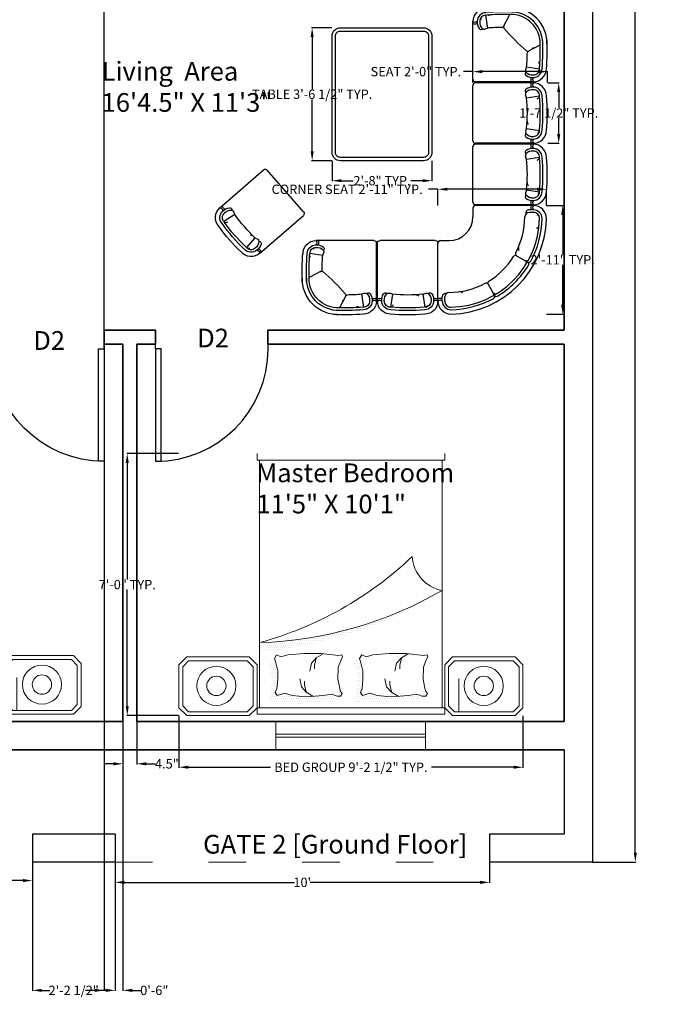
# Model space of a CAD drawing. Units: inches. Extents: x 593 to 1000, y 91 to 964.
# Tile 2 of 4: x 795 to 1000, y 91 to 406. Entities that reach past the tile are written whole.
import ezdxf

# ---------------------------------------------------------------- set-up
doc = ezdxf.new("R2010")
doc.units = ezdxf.units.IN
doc.header["$MEASUREMENT"] = 0
doc.linetypes.add('ACAD_ISO03W100', pattern=[30, 12, -18])
for name, color, linetype, lineweight in [('A-ANNO-DIMS', 2, 'Continuous', 13), ('A-ANNO-TEXT', 7, 'Continuous', 18), ('A-AREA-IDEN', 7, 'Continuous', 18), ('A-DOOR', 4, 'Continuous', 25), ('A-GLAZ', 4, 'Continuous', 18), ('A-WALL', 7, 'Continuous', 35), ('C-PROP', 7, 'Continuous', 30), ('C-SITE-GATE', 7, 'ACAD_ISO03W100', 18), ('FUR', 8, 'Continuous', 18)]:
    doc.layers.add(name, color=color, linetype=linetype, lineweight=lineweight)
doc.layers.add('ID-LOOSE', color=31, linetype='Continuous')
doc.layers.add('ID-LOOSE2', color=8, linetype='Continuous')
doc.styles.get("Standard").update_dxf_attribs({"font": 'arial.ttf'})
doc.dimstyles.get("Standard").update_dxf_attribs({"dimtxt": 3, "dimasz": 3, "dimexe": 0.18, "dimexo": 0.0625, "dimgap": 0.09, "dimtad": 0, "dimtih": 1, "dimtoh": 1, "dimdec": 1, "dimzin": 0, "dimdsep": 46, "dimlunit": 3, "dimtxsty": 'Standard', "dimcen": 0.09, "dimadec": 0, "dimazin": 0, "dimtfac": 1, "dimtdec": 1, "dimtofl": 0, "dimtmove": 0, "dimatfit": 3, "dimfxl": 1, "dimtolj": 1, "dimtzin": 0, "dimarcsym": 0})
pattern_1 = [(360, (-204.55691, -125.780183), (0.0079375, 0.015875), [0, -0.015875])]

# ---------------------------------------------------------------- blocks, each defined once
blk = doc.blocks.new('*U5')
for p, q in [((0, 0), (0, 6)), ((36, 0), (36, 6))]:
    blk.add_line(p, q)
blk.add_lwpolyline([(0, 0), (0, -36), (1.75, -36), (1.75, 0)], close=True)
blk.add_arc((0, 0), 36, 270, 0)
blk = doc.blocks.new('A$C9d18b682')
h = blk.add_hatch()
h.set_pattern_fill('DOTS', color=256, scale=0.01, style=0)
h.set_pattern_definition(pattern_1)
h.paths.add_polyline_path([(1.2038, 1.8915), (1.1915, 1.9099), (1.1638, 1.9099), (1.1238, 1.8945), (1.0562, 1.9068), (0.927, 1.916), (0.8193, 1.9068), (0.7639, 1.8884), (0.7055, 1.9068), (0.6901, 1.8822), (0.7024, 1.8546), (0.7086, 1.7839), (0.7086, 1.7163), (0.6932, 1.6548), (0.6839, 1.621), (0.6993, 1.5933), (0.7332, 1.6087), (0.7433, 1.6057), (0.7585, 1.6664), (0.7585, 1.734), (0.7523, 1.8047), (0.74, 1.8324), (0.7554, 1.857), (0.8139, 1.8385), (0.8692, 1.857), (0.9769, 1.8662), (1.1061, 1.857), (1.1738, 1.8447), (1.1846, 1.8488), (1.1884, 1.8699)])
h.paths.add_polyline_path([(1.8571, 1.8915), (1.8448, 1.9099), (1.8171, 1.9099), (1.7771, 1.8945), (1.7095, 1.9068), (1.5803, 1.916), (1.4726, 1.9068), (1.4172, 1.8884), (1.3588, 1.9068), (1.3434, 1.8822), (1.3557, 1.8546), (1.3618, 1.7839), (1.3618, 1.7163), (1.3465, 1.6548), (1.3372, 1.621), (1.3526, 1.5933), (1.3865, 1.6087), (1.3966, 1.6057), (1.4118, 1.6664), (1.4118, 1.734), (1.4056, 1.8047), (1.3933, 1.8324), (1.4087, 1.857), (1.4672, 1.8385), (1.5225, 1.857), (1.6302, 1.8662), (1.7594, 1.857), (1.8271, 1.8447), (1.8379, 1.8488), (1.8417, 1.8699)])
h = blk.add_hatch()
h.set_pattern_fill('DOTS', color=256, scale=0.01, style=0)
h.set_pattern_definition(pattern_1)
h.paths.add_polyline_path([(0.62, 1.5186), (0.62, 1.45, -0.124273), (2.02, 1.05, 0.122563)])
for p, q in [((2.04, 2), (0.6, 2)), ((0.6, 1.95), (0.6, 2)), ((2.04, 2), (2.04, 1.95)), ((2.1476, 1.9789), (2.1476, 1.7289)), ((2.04, 1.95), (0.6, 1.95)), ((0.62, 0.05), (0.62, 1.95)), ((2.02, 1.95), (2.02, 0.05)), ((2.04, 0.05), (0.6, 0.05)), ((0.6, 0), (0.6, 0.05)), ((2.04, 0.05), (2.04, 0))]:
    blk.add_line(p, q)
for points in [[(0.06, 1.56), (0.54, 1.56), (0.6, 1.62), (0.6, 1.95), (0.54, 2.01), (0.06, 2.01), (0, 1.95), (0, 1.62)], [(0.075, 1.59), (0.525, 1.59), (0.57, 1.635), (0.57, 1.935), (0.525, 1.98), (0.075, 1.98), (0.03, 1.935), (0.03, 1.635)], [(2.1, 1.56), (2.58, 1.56), (2.64, 1.62), (2.64, 1.95), (2.58, 2.01), (2.1, 2.01), (2.04, 1.95), (2.04, 1.62)], [(2.115, 1.59), (2.565, 1.59), (2.61, 1.635), (2.61, 1.935), (2.565, 1.98), (2.115, 1.98), (2.07, 1.935), (2.07, 1.635)]]:
    blk.add_lwpolyline(points, close=True)
for points in [[(0.8139, 1.8385), (0.7554, 1.857), (0.74, 1.8324), (0.7523, 1.8047), (0.7585, 1.734), (0.7585, 1.6664), (0.7431, 1.6049), (0.7339, 1.5711), (0.7493, 1.5434), (0.7831, 1.5588), (0.8354, 1.5434), (0.9615, 1.5342), (1.0907, 1.5342), (1.2261, 1.5496), (1.2507, 1.5434), (1.2568, 1.5588), (1.2445, 1.5834), (1.223, 1.6387), (1.2199, 1.7309), (1.2322, 1.7863), (1.2384, 1.8201), (1.2538, 1.8416), (1.2414, 1.86), (1.2138, 1.86), (1.1738, 1.8447), (1.1061, 1.857), (0.9769, 1.8662), (0.8692, 1.857), (0.8139, 1.8385)], [(1.0292, 1.86), (0.9769, 1.8293), (0.94, 1.7893), (0.9277, 1.7279)], [(0.9769, 1.8262), (0.9646, 1.777), (0.9646, 1.7463)], [(1.4672, 1.8385), (1.4087, 1.857), (1.3933, 1.8324), (1.4056, 1.8047), (1.4118, 1.734), (1.4118, 1.6664), (1.3964, 1.6049), (1.3872, 1.5711), (1.4026, 1.5434), (1.4364, 1.5588), (1.4887, 1.5434), (1.6148, 1.5342), (1.744, 1.5342), (1.8794, 1.5496), (1.904, 1.5434), (1.9101, 1.5588), (1.8978, 1.5834), (1.8763, 1.6387), (1.8732, 1.7309), (1.8855, 1.7863), (1.8917, 1.8201), (1.907, 1.8416), (1.8947, 1.86), (1.8671, 1.86), (1.8271, 1.8447), (1.7594, 1.857), (1.6302, 1.8662), (1.5225, 1.857), (1.4672, 1.8385)], [(1.6825, 1.86), (1.6302, 1.8293), (1.5933, 1.7893), (1.581, 1.7279)], [(1.6302, 1.8262), (1.6179, 1.777), (1.6179, 1.7463)], [(1.1061, 1.5373), (1.0538, 1.568), (1.0169, 1.608), (1.0046, 1.6695)], [(1.7594, 1.5373), (1.7071, 1.568), (1.6702, 1.608), (1.6579, 1.6695)], [(1.0538, 1.5711), (1.0415, 1.6203), (1.0415, 1.651)], [(1.7071, 1.5711), (1.6948, 1.6203), (1.6948, 1.651)]]:
    blk.add_lwpolyline(points)
for centre, radius in [((0.288, 1.782), 0.15), ((2.3392, 1.782), 0.15), ((0.288, 1.782), 0.0743), ((2.3392, 1.782), 0.0743)]:
    blk.add_circle(centre, radius)
for centre, radius, start, end in [((0.5277, -1.5229), 2.9743, 59.8866, 88.22261), ((-0.1045, -1.2025), 2.7497, 46.43667, 74.72336), ((2.0704, 0.7742), 0.2804, 100.35432, 176.78617)]:
    blk.add_arc(centre, radius, start, end)
blk = doc.blocks.new('A$C68294616')
at = {"layer": 'ID-LOOSE'}
for p, q in [((0.372, -0.31), (0.372, 0.36)), ((0.402, 0.39), (1.042, 0.39)), ((1.072, -0.31), (1.072, 0.36)), ((0.545, -0.231), (0.511, -0.219)), ((0.899, -0.231), (0.933, -0.219))]:
    blk.add_line(p, q, dxfattribs=at)
for centre, radius, start, end in [((0.402, 0.36), 0.03, 90, 180), ((1.042, 0.36), 0.03, 360, 90), ((0.554, -0.3), 0.133, 146.0897, 185.6132), ((0.465, -0.24), 0.025, 62.9608, 146.0897), ((0.452, -0.265), 0.0532, 51.0017, 62.9608), ((0.502, -0.242), 0.025, 70, 132.0066), ((0.942, -0.242), 0.025, 47.9934, 110), ((0.992, -0.265), 0.0532, 117.0392, 128.9983), ((0.979, -0.24), 0.025, 33.9103, 117.0392), ((0.89, -0.3), 0.133, 354.3868, 33.9103), ((0.397, -0.346), 0.0662, 67.8298, 112.1702), ((0.522, -0.31), 0.15, 180, 271.1754), ((0.522, -0.31), 0.1, 180, 271.1754), ((0.722, 1.538), 1.778, 264.2835, 275.7165), ((0.628, -0.286), 0.0481, 90.6237, 136.1803), ((0.922, -0.31), 0.15, 268.8246, 360), ((0.922, -0.31), 0.1, 268.8246, 360), ((1.047, -0.346), 0.0662, 67.8298, 112.1702), ((0.529, -0.332), 0.0481, 216.0775, 261.6341), ((0.722, 1.538), 1.958, 264.2835, 275.7165), ((0.933, -0.336), 0.0481, 201.2156, 246.7721), ((0.722, 1.538), 2.008, 264.2835, 275.7165)]:
    blk.add_arc(centre, radius, start, end, dxfattribs=at)
at = {"layer": 'ID-LOOSE2'}
for p, q in [((0.545, -0.231), (0.522, -0.38)), ((0.899, -0.231), (0.922, -0.38))]:
    blk.add_line(p, q, dxfattribs=at)
for centre, radius, start, end in [((0.554, -0.3), 0.103, 132.0066, 185.6132), ((0.89, -0.3), 0.103, 354.3868, 47.9934), ((0.397, -0.336), 0.0362, 46.3972, 133.6028), ((0.522, -0.31), 0.07, 180, 271.1754), ((0.922, -0.31), 0.07, 268.8246, 360), ((1.047, -0.336), 0.0362, 46.3972, 133.6028), ((0.722, 1.538), 1.928, 264.2835, 275.7165)]:
    blk.add_arc(centre, radius, start, end, dxfattribs=at)
blk = doc.blocks.new('A$C68FE3AF0')
at = {"layer": 'ID-LOOSE'}
for p, q in [((0.372, -0.31), (0.372, 0.36)), ((0.402, 0.39), (1.072, 0.39)), ((0.993, 0.217), (0.981, 0.251)), ((0.545, -0.231), (0.511, -0.219))]:
    blk.add_line(p, q, dxfattribs=at)
for centre, radius, start, end in [((0.402, 0.36), 0.03, 90, 180), ((1.098, 0.365), 0.0562, 153.6122, 206.6666), ((1.072, 0.24), 0.15, 358.8246, 90), ((1.002, 0.297), 0.025, 123.9103, 207.0392), ((1.004, 0.26), 0.025, 137.9934, 200), ((1.027, 0.31), 0.0532, 207.0392, 218.9983), ((1.062, 0.208), 0.133, 84.3868, 123.9103), ((1.072, 0.24), 0.1, 358.8246, 90), ((1.111, 0.29), 0.0136, 109.4209, 182.5668), ((1.121, 0.22), 0.0246, 302.8172, 29.8385), ((-0.776, 0.04), 1.958, 355.8657, 5.7165), ((-0.776, 0.04), 2.008, 355.818, 5.7165), ((-0.776, 0.04), 1.778, 0.3836, 5.7165), ((2.592, -1.83), 2.454, 130.6961, 139.3039), ((1.005, 0.016), 0.02, 62, 130.6961), ((1.022, 0.052), 0.02, 180.3836, 242), ((0.812, -0.05), 0.419, 268.2181, 1.7819), ((0.812, -0.05), 0.369, 268.2181, 1.7819), ((0.554, -0.3), 0.133, 146.0897, 185.6132), ((0.465, -0.24), 0.025, 62.9608, 146.0897), ((0.452, -0.265), 0.0532, 51.0017, 62.9608), ((0.502, -0.242), 0.025, 70, 132.0066), ((0.397, -0.336), 0.0562, 63.3334, 116.3878), ((0.522, -0.31), 0.15, 180, 271.1754), ((0.522, -0.31), 0.1, 180, 271.1754), ((0.722, 1.538), 1.778, 264.2835, 269.6164), ((0.71, -0.26), 0.02, 28, 89.6164), ((0.746, -0.243), 0.02, 139.3039, 208), ((0.786, -0.309), 0.0246, 151.3726, 194.8832), ((0.788, -0.313), 0.0246, 151.3726, 194.8832), ((0.722, 1.538), 1.958, 264.2835, 274.1343), ((0.575, -0.358), 0.0246, 281.4741, 324.9847), ((0.581, -0.359), 0.0246, 281.4741, 324.9847), ((0.722, 1.538), 2.008, 264.2835, 274.182)]:
    blk.add_arc(centre, radius, start, end, dxfattribs=at)
at = {"layer": 'ID-LOOSE2'}
for p, q in [((0.993, 0.217), (1.142, 0.24)), ((1.013, 0.034), (1.15, -0.039)), ((0.545, -0.231), (0.522, -0.38)), ((0.728, -0.251), (0.801, -0.388))]:
    blk.add_line(p, q, dxfattribs=at)
for centre, radius, start, end in [((1.098, 0.365), 0.0362, 136.3972, 223.6028), ((1.062, 0.208), 0.103, 84.3868, 137.9934), ((1.072, 0.24), 0.07, 358.8246, 90), ((-0.776, 0.04), 1.928, 357.6546, 5.7165), ((0.812, -0.05), 0.339, 268.2181, 1.7819), ((0.554, -0.3), 0.103, 132.0066, 185.6132), ((0.397, -0.336), 0.0362, 46.3972, 133.6028), ((0.522, -0.31), 0.07, 180, 271.1754), ((0.722, 1.538), 1.928, 264.2835, 272.3454)]:
    blk.add_arc(centre, radius, start, end, dxfattribs=at)
blk = doc.blocks.new('A$C707258B2')
at = {"layer": 'ID-LOOSE'}
for p, q in [((0.404, 0.342), (1.074, 0.342)), ((0.404, 0.292), (0.454, 0.292)), ((1.104, 0.312), (1.104, 0.212)), ((1.479, -0.063), (1.379, -0.063)), ((1.509, -0.763), (1.509, -0.093)), ((1.459, -0.763), (1.459, -0.712))]:
    blk.add_line(p, q, dxfattribs=at)
for centre, radius, start, end in [((0.404, 0.192), 0.15, 90, 181.1754), ((0.368, 0.317), 0.0662, 337.8298, 22.1702), ((1.074, 0.312), 0.03, 360, 90), ((0.404, 0.192), 0.1, 90, 181.1754), ((0.455, 0.256), 0.0357, 345.4262, 90.5555), ((0.454, 0.212), 0.05, 360, 90), ((1.379, 0.212), 1.125, 181.1754, 268.8246), ((1.379, 0.212), 1.075, 181.1754, 208.6357), ((1.379, 0.212), 0.875, 180, 208.4082), ((1.379, 0.212), 0.275, 180, 270), ((0.419, 0.102), 0.0935, 329.1864, 354.4231), ((1.479, -0.093), 0.03, 360, 90), ((0.587, -0.216), 0.025, 300, 28.4082), ((0.457, -0.291), 0.025, 208.6357, 300), ((0.482, -0.334), 0.025, 120, 211.3643), ((0.461, -0.295), 0.0199, 309.2667, 10.0983), ((0.481, -0.329), 0.0199, 49.9017, 110.7333), ((0.612, -0.259), 0.025, 31.5918, 120), ((1.379, 0.212), 0.875, 211.5918, 238.4082), ((1.379, 0.212), 1.075, 211.3643, 238.6357), ((0.907, -0.555), 0.025, 330, 58.4082), ((0.951, -0.58), 0.025, 61.5918, 150), ((1.379, 0.212), 0.875, 241.5918, 270), ((0.838, -0.686), 0.0199, 339.2667, 40.0983), ((1.019, -0.683), 0.0935, 84.0982, 109.3349), ((1.379, -0.713), 0.05, 360, 90), ((1.425, -0.709), 0.0336, 354.6301, 109.3883), ((0.832, -0.685), 0.025, 238.6357, 330), ((0.876, -0.71), 0.025, 150, 241.3643), ((0.872, -0.706), 0.0199, 79.9017, 140.7333), ((1.379, 0.212), 1.075, 241.3643, 268.8246), ((1.359, -0.763), 0.15, 268.8246, 360), ((1.359, -0.763), 0.1, 268.8246, 360), ((1.484, -0.799), 0.0662, 67.8298, 112.1702), ((1.291, -0.783), 0.0481, 201.2156, 246.7721), ((1.405, -0.803), 0.00999, 211.067, 288.5313)]:
    blk.add_arc(centre, radius, start, end, dxfattribs=at)
at = {"layer": 'ID-LOOSE2'}
for p, q in [((0.404, 0.262), (0.454, 0.262)), ((0.6, -0.238), (0.47, -0.313)), ((0.929, -0.567), (0.854, -0.697)), ((1.429, -0.763), (1.429, -0.713))]:
    blk.add_line(p, q, dxfattribs=at)
for centre, radius, start, end in [((0.378, 0.317), 0.0362, 316.3972, 43.6028), ((0.404, 0.192), 0.07, 90, 181.1754), ((1.379, 0.212), 1.045, 181.1754, 268.8246), ((1.359, -0.763), 0.07, 268.8246, 360), ((1.484, -0.789), 0.0362, 46.3972, 133.6028)]:
    blk.add_arc(centre, radius, start, end, dxfattribs=at)
blk = doc.blocks.new('A$C1352')
at = {"layer": 'ID-LOOSE'}
blk.add_lwpolyline([(0.0027, 0.053), (0.0027, 0.553, -0.414214), (0.0527, 0.603), (0.7527, 0.603, -0.414214), (0.8027, 0.553), (0.8027, 0.053, -0.414214), (0.7527, 0.003), (0.0527, 0.003, -0.414214)], format="xyb", close=True, dxfattribs=at)
at = {"layer": 'ID-LOOSE2'}
blk.add_lwpolyline([(0.0227, 0.053), (0.0227, 0.553, -0.414214), (0.0527, 0.583), (0.7527, 0.583, -0.414214), (0.7827, 0.553), (0.7827, 0.053, -0.414214), (0.7527, 0.023), (0.0527, 0.023, -0.414214)], format="xyb", close=True, dxfattribs=at)
blk = doc.blocks.new('*D15')
at = {"layer": 'A-ANNO-DIMS', "color": 0, "lineweight": -2, "transparency": 16777216}
for p, q in [((678.91, 136.12), (678.91, 130.08)), ((798.91, 136.12), (798.91, 130.08)), ((681.91, 130.26), (736.42, 130.26)), ((795.91, 130.26), (741.4, 130.26))]:
    blk.add_line(p, q, dxfattribs=at)
at = {"layer": 'A-ANNO-DIMS', "color": 0, "transparency": 16777216}
for points in [[(681.91, 130.76), (681.91, 129.76), (678.91, 130.26)], [(795.91, 130.76), (795.91, 129.76), (798.91, 130.26)]]:
    blk.add_solid(points, dxfattribs=at)
at = {"layer": 'Defpoints', "color": 0, "transparency": 16777216}
for p in [(678.91, 136.18), (798.91, 136.18), (798.91, 130.26)]:
    blk.add_point(p, dxfattribs=at)
at = {"layer": 'A-ANNO-DIMS', "color": 0, "transparency": 16777216, "insert": (738.91, 130.26), "char_height": 3, "attachment_point": 5}
blk.add_mtext("\\A1;10'", dxfattribs=at)
blk = doc.blocks.new('*D16')
at = {"layer": 'A-ANNO-DIMS', "color": 0, "lineweight": -2, "transparency": 16777216}
for p, q in [((825.41, 136.12), (825.41, 129.51)), ((945.41, 136.12), (945.41, 129.51)), ((828.41, 129.69), (882.92, 129.69)), ((942.41, 129.69), (887.9, 129.69))]:
    blk.add_line(p, q, dxfattribs=at)
at = {"layer": 'A-ANNO-DIMS', "color": 0, "transparency": 16777216}
for points in [[(828.41, 130.19), (828.41, 129.19), (825.41, 129.69)], [(942.41, 130.19), (942.41, 129.19), (945.41, 129.69)]]:
    blk.add_solid(points, dxfattribs=at)
at = {"layer": 'Defpoints', "color": 0, "transparency": 16777216}
for p in [(825.41, 136.18), (945.41, 136.18), (945.41, 129.69)]:
    blk.add_point(p, dxfattribs=at)
at = {"layer": 'A-ANNO-DIMS', "color": 0, "transparency": 16777216, "insert": (885.41, 129.69), "char_height": 3, "attachment_point": 5}
blk.add_mtext("\\A1;10'", dxfattribs=at)
blk = doc.blocks.new('*D18')
at = {"layer": 'A-ANNO-DIMS', "color": 0, "lineweight": -2, "transparency": 16777216}
for p, q in [((827.91, 181.12), (827.91, 167.5)), ((832.41, 181.12), (832.41, 167.5)), ((824.91, 167.68), (821.91, 167.68)), ((835.41, 167.68), (838.41, 167.68))]:
    blk.add_line(p, q, dxfattribs=at)
at = {"layer": 'A-ANNO-DIMS', "color": 0, "transparency": 16777216}
for points in [[(824.91, 168.18), (824.91, 167.18), (827.91, 167.68)], [(835.41, 168.18), (835.41, 167.18), (832.41, 167.68)]]:
    blk.add_solid(points, dxfattribs=at)
at = {"layer": 'Defpoints', "color": 0, "transparency": 16777216}
for p in [(827.91, 181.18), (832.41, 181.18), (832.41, 167.68)]:
    blk.add_point(p, dxfattribs=at)
at = {"layer": 'A-ANNO-DIMS', "color": 0, "transparency": 16777216, "insert": (842.03, 167.68), "char_height": 3, "attachment_point": 5}
blk.add_mtext('\\A1;4.5"', dxfattribs=at)
blk = doc.blocks.new('*D29')
at = {"layer": 'A-ANNO-DIMS', "color": 0, "lineweight": -2, "transparency": 16777216}
for p, q in [((978.47, 920.68), (992.35, 920.68)), ((992.17, 917.68), (992.17, 530.06)), ((992.17, 139.18), (992.17, 526.81)), ((978.47, 136.18), (992.35, 136.18))]:
    blk.add_line(p, q, dxfattribs=at)
at = {"layer": 'A-ANNO-DIMS', "color": 0, "transparency": 16777216}
for points in [[(991.67, 917.68), (992.67, 917.68), (992.17, 920.68)], [(991.67, 139.18), (992.67, 139.18), (992.17, 136.18)]]:
    blk.add_solid(points, dxfattribs=at)
at = {"layer": 'Defpoints', "color": 0, "transparency": 16777216}
for p in [(978.41, 920.68), (992.17, 920.68), (978.41, 136.18)]:
    blk.add_point(p, dxfattribs=at)
at = {"layer": 'A-ANNO-DIMS', "color": 0, "transparency": 16777216, "insert": (992.17, 528.43), "char_height": 3, "attachment_point": 5}
blk.add_mtext('\\A1;65\'-4.5"', dxfattribs=at)
blk = doc.blocks.new('WIN-48')
for p, q in [((0, 0), (0, 9)), ((48, 0), (48, 9)), ((0, 5), (48, 5)), ((0, 4), (48, 4))]:
    blk.add_line(p, q)
blk = doc.blocks.new('*D40')
at = {"layer": 'A-ANNO-DIMS', "color": 0, "lineweight": -2, "transparency": 16777216}
for p, q in [((845.86, 183.06), (845.86, 166.4)), ((956.15, 183.06), (956.15, 166.4)), ((848.86, 166.58), (875.19, 166.58)), ((953.15, 166.58), (926.83, 166.58))]:
    blk.add_line(p, q, dxfattribs=at)
at = {"layer": 'A-ANNO-DIMS', "color": 0, "transparency": 16777216}
for points in [[(848.86, 167.08), (848.86, 166.08), (845.86, 166.58)], [(953.15, 167.08), (953.15, 166.08), (956.15, 166.58)]]:
    blk.add_solid(points, dxfattribs=at)
at = {"layer": 'Defpoints', "color": 0, "transparency": 16777216}
for p in [(845.86, 183.12), (956.15, 183.12), (956.15, 166.58)]:
    blk.add_point(p, dxfattribs=at)
at = {"layer": 'A-ANNO-DIMS', "color": 0, "transparency": 16777216, "insert": (901.01, 166.58), "char_height": 3, "attachment_point": 5}
blk.add_mtext('\\A1;BED GROUP 9\'-2 1/2" TYP.', dxfattribs=at)
blk = doc.blocks.new('*D41')
at = {"layer": 'A-ANNO-DIMS', "color": 0, "lineweight": -2, "transparency": 16777216}
for p, q in [((845.8, 267.1), (829.14, 267.1)), ((829.32, 264.1), (829.32, 226.73)), ((829.32, 186.12), (829.32, 223.49)), ((845.8, 183.12), (829.14, 183.12))]:
    blk.add_line(p, q, dxfattribs=at)
at = {"layer": 'A-ANNO-DIMS', "color": 0, "transparency": 16777216}
for points in [[(828.82, 264.1), (829.82, 264.1), (829.32, 267.1)], [(828.82, 186.12), (829.82, 186.12), (829.32, 183.12)]]:
    blk.add_solid(points, dxfattribs=at)
at = {"layer": 'Defpoints', "color": 0, "transparency": 16777216}
for p in [(845.86, 267.1), (829.32, 183.12), (845.86, 183.12)]:
    blk.add_point(p, dxfattribs=at)
at = {"layer": 'A-ANNO-DIMS', "color": 0, "transparency": 16777216, "insert": (829.32, 225.11), "char_height": 3, "attachment_point": 5}
blk.add_mtext('\\A1;7\'-0" TYP.', dxfattribs=at)
blk = doc.blocks.new('*D42')
at = {"layer": 'A-ANNO-DIMS', "color": 0, "lineweight": -2, "transparency": 16777216}
for p, q in [((940.11, 389.47), (937.11, 389.47)), ((940.11, 385.95), (940.11, 389.65)), ((961.02, 389.47), (943.11, 389.47)), ((964.02, 385.95), (964.02, 389.65))]:
    blk.add_line(p, q, dxfattribs=at)
at = {"layer": 'A-ANNO-DIMS', "color": 0, "transparency": 16777216}
for points in [[(943.11, 389.97), (943.11, 388.97), (940.11, 389.47)], [(961.02, 389.97), (961.02, 388.97), (964.02, 389.47)]]:
    blk.add_solid(points, dxfattribs=at)
at = {"layer": 'Defpoints', "color": 0, "transparency": 16777216}
for p in [(940.11, 389.47), (940.11, 385.89), (964.02, 385.89)]:
    blk.add_point(p, dxfattribs=at)
at = {"layer": 'A-ANNO-DIMS', "color": 0, "transparency": 16777216, "insert": (921.83, 389.47), "char_height": 3, "attachment_point": 5}
blk.add_mtext('\\A1;SEAT 2\'-0" TYP.', dxfattribs=at)
blk = doc.blocks.new('*D43')
at = {"layer": 'A-ANNO-DIMS', "color": 0, "lineweight": -2, "transparency": 16777216}
for p, q in [((964.08, 385.89), (967.79, 385.89)), ((967.61, 382.89), (967.61, 377.83)), ((967.61, 369.5), (967.61, 374.55)), ((964.08, 366.5), (967.79, 366.5))]:
    blk.add_line(p, q, dxfattribs=at)
at = {"layer": 'A-ANNO-DIMS', "color": 0, "transparency": 16777216}
for points in [[(967.11, 382.89), (968.11, 382.89), (967.61, 385.89)], [(967.11, 369.5), (968.11, 369.5), (967.61, 366.5)]]:
    blk.add_solid(points, dxfattribs=at)
at = {"layer": 'Defpoints', "color": 0, "transparency": 16777216}
for p in [(964.02, 385.89), (967.61, 385.89), (964.02, 366.5)]:
    blk.add_point(p, dxfattribs=at)
at = {"layer": 'A-ANNO-DIMS', "color": 0, "transparency": 16777216, "insert": (967.61, 376.19), "char_height": 3, "attachment_point": 5}
blk.add_mtext('\\A1;1\'-7 1/2" TYP.', dxfattribs=at)
blk = doc.blocks.new('*D46')
at = {"layer": 'A-ANNO-DIMS', "color": 0, "lineweight": -2, "transparency": 16777216}
for p, q in [((928.9, 351.77), (925.9, 351.77)), ((928.9, 346.62), (928.9, 351.95)), ((960.67, 351.77), (931.9, 351.77)), ((963.67, 346.62), (963.67, 351.95))]:
    blk.add_line(p, q, dxfattribs=at)
at = {"layer": 'A-ANNO-DIMS', "color": 0, "transparency": 16777216}
for points in [[(931.9, 352.27), (931.9, 351.27), (928.9, 351.77)], [(960.67, 352.27), (960.67, 351.27), (963.67, 351.77)]]:
    blk.add_solid(points, dxfattribs=at)
at = {"layer": 'Defpoints', "color": 0, "transparency": 16777216}
for p in [(928.9, 351.77), (928.9, 346.56), (963.67, 346.56)]:
    blk.add_point(p, dxfattribs=at)
at = {"layer": 'A-ANNO-DIMS', "color": 0, "transparency": 16777216, "insert": (899.8, 351.77), "char_height": 3, "attachment_point": 5}
blk.add_mtext('\\A1;CORNER SEAT 2\'-11" TYP.', dxfattribs=at)
blk = doc.blocks.new('*D47')
at = {"layer": 'A-ANNO-DIMS', "color": 0, "lineweight": -2, "transparency": 16777216}
for p, q in [((963.74, 346.56), (969.07, 346.56)), ((968.89, 343.56), (968.89, 330.76)), ((968.89, 314.78), (968.89, 327.57)), ((963.74, 311.78), (969.07, 311.78))]:
    blk.add_line(p, q, dxfattribs=at)
at = {"layer": 'A-ANNO-DIMS', "color": 0, "transparency": 16777216}
for points in [[(968.39, 343.56), (969.39, 343.56), (968.89, 346.56)], [(968.39, 314.78), (969.39, 314.78), (968.89, 311.78)]]:
    blk.add_solid(points, dxfattribs=at)
at = {"layer": 'Defpoints', "color": 0, "transparency": 16777216}
for p in [(963.67, 346.56), (968.89, 346.56), (963.67, 311.78)]:
    blk.add_point(p, dxfattribs=at)
at = {"layer": 'A-ANNO-DIMS', "color": 0, "transparency": 16777216, "insert": (968.89, 329.17), "char_height": 3, "attachment_point": 5}
blk.add_mtext('\\A1;2\'-11" TYP.', dxfattribs=at)
blk = doc.blocks.new('*D48')
at = {"layer": 'A-ANNO-DIMS', "color": 0, "lineweight": -2, "transparency": 16777216}
for p, q in [((894.92, 403.54), (888.41, 403.54)), ((888.59, 400.54), (888.59, 383.87)), ((888.59, 363.91), (888.59, 380.58)), ((894.92, 360.91), (888.41, 360.91))]:
    blk.add_line(p, q, dxfattribs=at)
at = {"layer": 'A-ANNO-DIMS', "color": 0, "transparency": 16777216}
for points in [[(888.09, 400.54), (889.09, 400.54), (888.59, 403.54)], [(888.09, 363.91), (889.09, 363.91), (888.59, 360.91)]]:
    blk.add_solid(points, dxfattribs=at)
at = {"layer": 'Defpoints', "color": 0, "transparency": 16777216}
for p in [(888.59, 403.54), (894.99, 403.54), (894.99, 360.91)]:
    blk.add_point(p, dxfattribs=at)
at = {"layer": 'A-ANNO-DIMS', "color": 0, "transparency": 16777216, "insert": (888.59, 382.23), "char_height": 3, "attachment_point": 5}
blk.add_mtext('\\A1;TABLE 3\'-6 1/2" TYP.', dxfattribs=at)
blk = doc.blocks.new('*D49')
at = {"layer": 'A-ANNO-DIMS', "color": 0, "lineweight": -2, "transparency": 16777216}
for p, q in [((894.99, 360.85), (894.99, 354.34)), ((926.96, 360.85), (926.96, 354.34)), ((897.99, 354.52), (901.71, 354.52)), ((923.96, 354.52), (920.23, 354.52))]:
    blk.add_line(p, q, dxfattribs=at)
at = {"layer": 'A-ANNO-DIMS', "color": 0, "transparency": 16777216}
for points in [[(897.99, 355.02), (897.99, 354.02), (894.99, 354.52)], [(923.96, 355.02), (923.96, 354.02), (926.96, 354.52)]]:
    blk.add_solid(points, dxfattribs=at)
at = {"layer": 'Defpoints', "color": 0, "transparency": 16777216}
for p in [(894.99, 360.91), (926.96, 360.91), (894.99, 354.52)]:
    blk.add_point(p, dxfattribs=at)
at = {"layer": 'A-ANNO-DIMS', "color": 0, "transparency": 16777216, "insert": (910.97, 354.52), "char_height": 3, "attachment_point": 5}
blk.add_mtext('\\A1;2\'-8" TYP.', dxfattribs=at)
blk = doc.blocks.new('*D55')
at = {"layer": 'A-ANNO-DIMS', "color": 0, "lineweight": -2, "transparency": 16777216}
for p, q in [((798.91, 136.12), (798.91, 94.9)), ((825.41, 136.12), (825.41, 94.9)), ((801.91, 95.08), (804.56, 95.08)), ((822.41, 95.08), (819.76, 95.08))]:
    blk.add_line(p, q, dxfattribs=at)
at = {"layer": 'A-ANNO-DIMS', "color": 0, "transparency": 16777216}
for points in [[(801.91, 95.58), (801.91, 94.58), (798.91, 95.08)], [(822.41, 95.58), (822.41, 94.58), (825.41, 95.08)]]:
    blk.add_solid(points, dxfattribs=at)
at = {"layer": 'Defpoints', "color": 0, "transparency": 16777216}
for p in [(798.91, 136.18), (825.41, 136.18), (825.41, 95.08)]:
    blk.add_point(p, dxfattribs=at)
at = {"layer": 'A-ANNO-DIMS', "color": 0, "transparency": 16777216, "insert": (812.16, 95.08), "char_height": 3, "attachment_point": 5}
blk.add_mtext('\\A1;2\'-2 1/2"', dxfattribs=at)
blk = doc.blocks.new('*D60')
at = {"layer": 'A-ANNO-DIMS', "color": 0, "lineweight": -2, "transparency": 16777216}
for p, q in [((785.91, 306.75), (785.91, 961.96)), ((788.91, 961.78), (799.83, 961.78)), ((818.91, 961.78), (807.99, 961.78)), ((821.91, 306.75), (821.91, 961.96))]:
    blk.add_line(p, q, dxfattribs=at)
at = {"layer": 'A-ANNO-DIMS', "color": 0, "transparency": 16777216}
for points in [[(788.91, 962.28), (788.91, 961.28), (785.91, 961.78)], [(818.91, 962.28), (818.91, 961.28), (821.91, 961.78)]]:
    blk.add_solid(points, dxfattribs=at)
at = {"layer": 'Defpoints', "color": 0, "transparency": 16777216}
for p in [(821.91, 961.78), (785.91, 306.68), (821.91, 306.68)]:
    blk.add_point(p, dxfattribs=at)
at = {"layer": 'A-ANNO-DIMS', "color": 0, "transparency": 16777216, "insert": (803.91, 961.78), "char_height": 3, "attachment_point": 5}
blk.add_mtext('\\A1;3\'-0"', dxfattribs=at)
blk = doc.blocks.new('*D63')
at = {"layer": 'A-ANNO-DIMS', "color": 0, "lineweight": -2, "transparency": 16777216}
for p, q in [((821.91, 302.12), (821.91, 94.9)), ((827.91, 302.12), (827.91, 94.9)), ((818.91, 95.08), (815.91, 95.08)), ((830.91, 95.08), (833.91, 95.08))]:
    blk.add_line(p, q, dxfattribs=at)
at = {"layer": 'A-ANNO-DIMS', "color": 0, "transparency": 16777216}
for points in [[(818.91, 95.58), (818.91, 94.58), (821.91, 95.08)], [(830.91, 95.58), (830.91, 94.58), (827.91, 95.08)]]:
    blk.add_solid(points, dxfattribs=at)
at = {"layer": 'Defpoints', "color": 0, "transparency": 16777216}
for p in [(821.91, 302.18), (827.91, 302.18), (827.91, 95.08)]:
    blk.add_point(p, dxfattribs=at)
at = {"layer": 'A-ANNO-DIMS', "color": 0, "transparency": 16777216, "insert": (837.99, 95.08), "char_height": 3, "attachment_point": 5}
blk.add_mtext('\\A1;0\'-6"', dxfattribs=at)

msp = doc.modelspace()

# ---------------------------------------------------------------- linework, layer by layer
at = {"layer": 'A-WALL'}
for p, q in [((821.91, 302.18), (821.91, 306.68)), ((838.41, 306.68), (821.91, 306.68)), ((838.41, 302.18), (838.41, 306.68)), ((969.41, 306.68), (874.41, 306.68)), ((874.41, 302.18), (874.41, 306.68)), ((827.91, 302.18), (821.91, 302.18)), ((838.41, 302.18), (832.41, 302.18)), ((969.41, 302.18), (874.41, 302.18)), ((827.91, 181.18), (690.91, 181.18)), ((969.41, 181.18), (832.41, 181.18)), ((969.41, 172.18), (681.91, 172.18))]:
    msp.add_line(p, q, dxfattribs=at)
for points in [[(969.41, 441.68), (969.41, 306.68)], [(827.91, 302.18), (827.91, 181.18)], [(832.41, 302.18), (832.41, 181.18)], [(969.41, 302.18), (969.41, 181.18)]]:
    msp.add_lwpolyline(points, dxfattribs=at)
at = {"layer": 'C-PROP'}
for p, q in [((978.41, 920.68), (978.41, 136.18)), ((798.91, 145.18), (798.91, 136.18)), ((825.41, 145.18), (825.41, 136.18)), ((945.41, 145.18), (945.41, 136.18))]:
    msp.add_line(p, q, dxfattribs=at)
for points in [[(678.91, 136.18), (645.91, 136.18), (645.91, 920.68), (978.41, 920.68), (978.41, 136.18), (945.41, 136.18)], [(969.41, 172.18), (969.41, 145.18), (945.41, 145.18)], [(825.41, 145.18), (798.91, 145.18)], [(825.41, 136.18), (798.91, 136.18)]]:
    msp.add_lwpolyline(points, dxfattribs=at)
at = {"layer": 'C-SITE-GATE'}
for p, q in [((678.91, 136.18), (798.91, 136.18)), ((825.41, 136.18), (945.41, 136.18))]:
    msp.add_line(p, q, dxfattribs=at)

# ---------------------------------------------------------------- block references
at = {"layer": 'A-DOOR', "yscale": 1.001918595307477, "zscale": 1.001918595307477}
for p, xscale in [((821.91, 300.67), -1.001918595307477), ((838.41, 300.67), 1.001918595307477)]:
    msp.add_blockref('*U5', p, dxfattribs=dict(at, xscale=xscale))
at = {"layer": 'A-GLAZ', "rotation": 180}
msp.add_blockref('WIN-48', (924.91, 181.18), dxfattribs=at)
at = {"layer": 'FUR'}
for name, p, xscale, yscale, zscale, rotation in [('A$C68FE3AF0', (950.91, 375.9), 27.69884856456519, 27.69884856456519, 27.69884856456519, 90.00000000066171), ('A$C1352', (927.11, 360.77), 53.28214672932182, 53.28214672932182, 53.28214672932182, 90), ('A$C68294616', (950.91, 356.19), 27.69884856456519, 27.69884856456519, 27.69884856456519, 90.00000000066171), ('A$C68294616', (950.91, 336.52), 27.69884856456519, 27.69884856456519, 27.69884856456519, 90.00000000066171), ('A$C68294616', (885, 329.06), -27.69884856456519, 27.69884856456519, 27.69884856456519, 311.0000000006589), ('A$C707258B2', (938.37, 304.76), 27.69884856456519, 27.69884856456519, 27.69884856456519, 90.00000000066171), ('A$C9d18b682', (704.26, 267.51), -41.77713228862137, 41.77713228862137, 41.77713228862137, 179.9999999999977), ('A$C9d18b682', (845.86, 267.1), -41.77713228862137, 41.77713228862137, 41.77713228862137, 179.9999999999977)]:
    msp.add_blockref(name, p, dxfattribs=dict(at, xscale=xscale, yscale=yscale, zscale=zscale, rotation=rotation))
at = {"layer": 'FUR', "xscale": -27.69884856456519, "yscale": 27.69884856456519, "zscale": 27.69884856456519}
for name, p in [('A$C68FE3AF0', (919.5, 324.54)), ('A$C68294616', (939.2, 324.54))]:
    msp.add_blockref(name, p, dxfattribs=at)

# ---------------------------------------------------------------- texts
at = {"layer": 'A-ANNO-TEXT', "char_height": 6, "attachment_point": 1}
for s, width, insert in [('{D2}', 8.544, (799.2, 306.32)), ('{D2}', 8.544, (851.73, 307.1)), ('GATE 2 [Ground Floor]', 87.7828, (853.63, 144.9))]:
    msp.add_mtext_dynamic_manual_height_columns(s, width=width, gutter_width=1, heights=[0], dxfattribs=dict(at, insert=insert))
at = {"layer": 'A-AREA-IDEN', "char_height": 6, "attachment_point": 1}
for s, insert in [('Living  Area\\P16\'4.5" X 11\'3"', (821.11, 392.59)), ('Master Bedroom\\P11\'5" X 10\'1"', (870.73, 263.91))]:
    msp.add_mtext_dynamic_manual_height_columns(s, width=76.3054, gutter_width=1, heights=[0], dxfattribs=dict(at, insert=insert))

# ---------------------------------------------------------------- dimensions: what is measured, and where the dimension line sits
at = {"layer": 'A-ANNO-DIMS'}
for base, p1, p2, override, picture, middle in [((821.91, 961.78), (785.91, 306.68), (821.91, 306.68), {"dimdec": 1, "dimlfac": 1, "dimrnd": 0, "dimzin": 1, "dimdsep": 46, "dimlunit": 4, "dimfrac": 2}, '*D60', (803.91, 961.78)), ((827.91, 95.08), (821.91, 302.18), (827.91, 302.18), {"dimdec": 1, "dimlfac": 1, "dimrnd": 0, "dimzin": 1, "dimdsep": 46, "dimlunit": 4, "dimfrac": 2}, '*D63', (837.99, 95.08)), ((832.41, 167.68), (827.91, 181.18), (832.41, 181.18), {"dimclrd": 0, "dimclre": 0, "dimclrt": 0}, '*D18', (842.03, 167.68)), ((798.91, 130.26), (678.91, 136.18), (798.91, 136.18), {"dimclrd": 0, "dimclre": 0, "dimclrt": 0}, '*D15', (738.91, 130.26)), ((825.41, 95.08), (798.91, 136.18), (825.41, 136.18), {"dimdec": 1, "dimlfac": 1, "dimrnd": 0, "dimzin": 1, "dimdsep": 46, "dimlunit": 4, "dimfrac": 2}, '*D55', (812.16, 95.08)), ((945.41, 129.69), (825.41, 136.18), (945.41, 136.18), {"dimclrd": 0, "dimclre": 0, "dimclrt": 0}, '*D16', (885.41, 129.69))]:
    dim = msp.add_linear_dim(base=base, p1=p1, p2=p2, dimstyle='Standard', override=override, dxfattribs=at)
    dim.commit()
    dim.dimension.update_dxf_attribs({"geometry": picture, "text_midpoint": middle})
dim = msp.add_linear_dim(base=(992.17, 920.68), p1=(978.41, 136.18), p2=(978.41, 920.68), angle=90, dimstyle='Standard', override={"dimclrd": 0, "dimclre": 0, "dimclrt": 0}, dxfattribs=at)
dim.commit()
dim.dimension.update_dxf_attribs({"geometry": '*D29', "text_midpoint": (992.17, 528.43)})
for base, p1, p2, angle, text, picture, middle in [((888.59, 403.54), (894.99, 360.91), (894.99, 403.54), 90, 'TABLE <> TYP.', '*D48', (888.59, 382.23)), ((940.11, 389.47), (964.02, 385.89), (940.11, 385.89), 180, 'SEAT <> TYP.', '*D42', (921.83, 389.47)), ((967.61, 385.89), (964.02, 366.5), (964.02, 385.89), 90, '<> TYP.', '*D43', (967.61, 376.19)), ((928.9, 351.77), (963.67, 346.56), (928.9, 346.56), 180, 'CORNER SEAT <> TYP.', '*D46', (899.8, 351.77)), ((894.99, 354.52), (926.96, 360.91), (894.99, 360.91), 180, '<> TYP.', '*D49', (910.97, 354.52)), ((968.89, 346.56), (963.67, 311.78), (963.67, 346.56), 90, '<> TYP.', '*D47', (968.89, 329.17)), ((829.32, 183.12), (845.86, 267.1), (845.86, 183.12), 270, '<> TYP.', '*D41', (829.32, 225.11))]:
    dim = msp.add_linear_dim(base=base, p1=p1, p2=p2, angle=angle, text=text, dimstyle='Standard', override={"dimdec": 1, "dimlfac": 1, "dimrnd": 0, "dimzin": 1, "dimdsep": 46, "dimlunit": 4, "dimfrac": 2}, dxfattribs=at)
    dim.commit()
    dim.dimension.update_dxf_attribs({"geometry": picture, "text_midpoint": middle})
dim = msp.add_linear_dim(base=(956.15, 166.58), p1=(845.86, 183.12), p2=(956.15, 183.12), text='BED GROUP <> TYP.', dimstyle='Standard', override={"dimdec": 1, "dimlfac": 1, "dimrnd": 0, "dimzin": 1, "dimdsep": 46, "dimlunit": 4, "dimfrac": 2}, dxfattribs=at)
dim.commit()
dim.dimension.update_dxf_attribs({"geometry": '*D40', "text_midpoint": (901.01, 166.58)})

doc.saveas('drawing.dxf')
